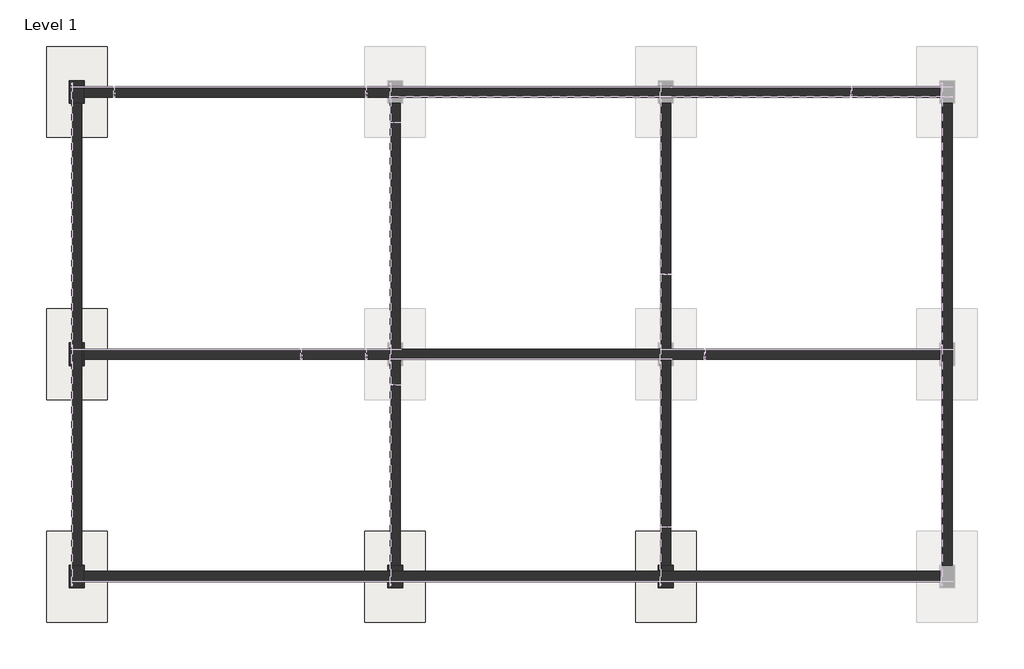
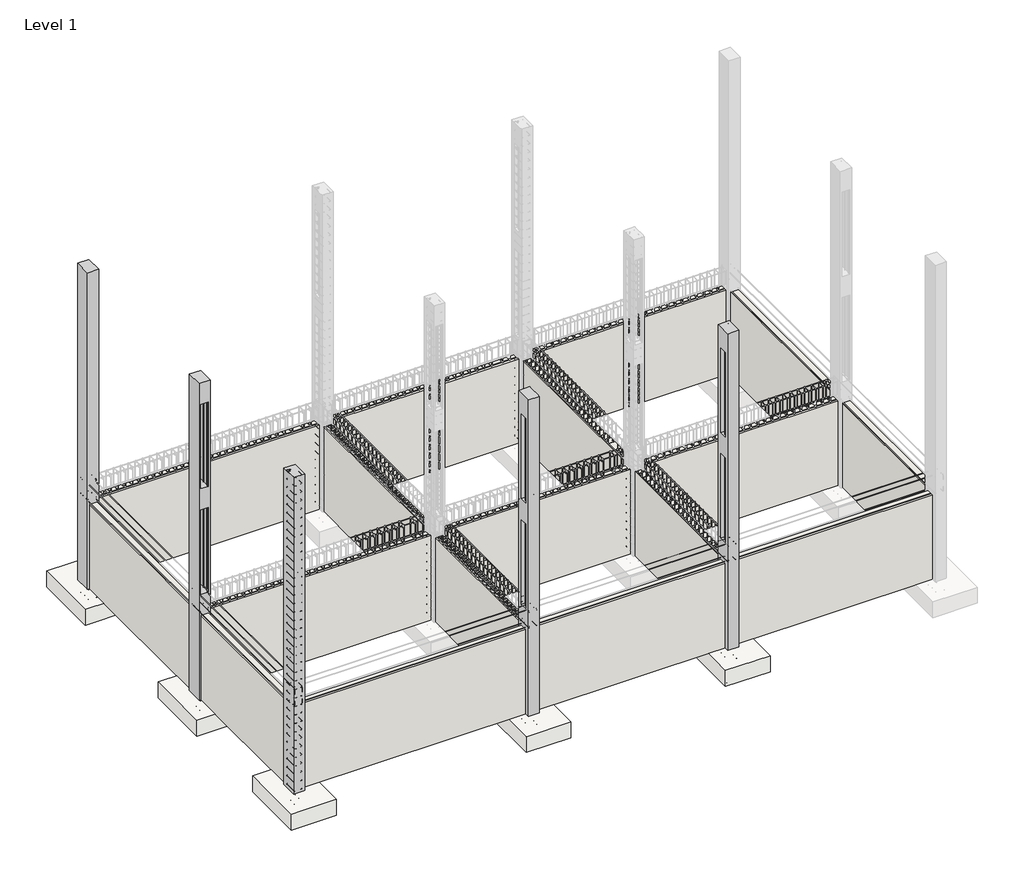
# One storey, part 1 of 8: 7 walls, 5 columns, 5 slabs.
"""IFC4 building model written with IfcOpenShell, lengths in millimetres."""

from ifc_helpers import new_model, si_unit, frame, origin, place, context, project, spatial, polyline, outline, extrude, faceted_brep, element, save

model = new_model("IFC4")

# Units and contexts
model_context = context("Model", 3, world=origin())
ifc_project = project(units=[si_unit("LENGTHUNIT", "METRE", prefix="MILLI")], contexts=[model_context])

# Site, building, storey
site = spatial("IfcSite", under=ifc_project)
building = spatial("IfcBuilding", under=site)
storey = spatial("IfcBuildingStorey", under=building, Name="Level 1", Elevation=0.0)

# Columns
placement = place(None, origin())
element("IfcColumn", 1, ObjectType="Concrete-Rectangular-Column : 12 x 18", at=placement, inside=storey, context=model_context, shape_type="Brep", body=[
    faceted_brep([(-20613.7343089, 13100.2555262, 0.0), (-20613.7343089, 12973.2555262, 0.0), (-20613.7343089, 12770.0555262, 0.0), (-20613.7343089, 12643.0555262, 0.0), (-20664.5343089, 12643.0555262, 0.0), (-20867.7343089, 12643.0555262, 0.0), (-20918.5343089, 12643.0555262, 0.0), (-20918.5343089, 13100.2555262, 0.0), (-20613.7343089, 13100.2555262, 9144.0), (-20613.7343089, 12643.0555262, 9144.0), (-20918.5343089, 12643.0555262, 9144.0), (-20918.5343089, 13100.2555262, 9144.0)], [[[0, 1, 2, 3, 4, 5, 6, 7]], [[8, 9, 3, 2, 1, 0]], [[9, 10, 6, 5, 4, 3]], [[10, 11, 7, 6]], [[11, 8, 0, 7]], [[8, 11, 10, 9]]]),
])
element("IfcColumn", 2, ObjectType="Concrete-Rectangular-Column : 12 x 18", at=placement, inside=storey, context=model_context, shape_type="Brep", body=[
    faceted_brep([(-20918.5343089, 7364.6820829, 0.0), (-20918.5343089, 7821.8820829, 0.0), (-20867.7343089, 7821.8820829, 0.0), (-20867.7343089, 7364.6820829, 0.0), (-20613.7343089, 7364.6820829, 0.0), (-20613.7343089, 7491.6820829, 0.0), (-20613.7343089, 7694.8820829, 0.0), (-20613.7343089, 7821.8820829, 0.0), (-20613.7343089, 7821.8820829, 2438.4), (-20613.7343089, 7821.8820829, 3048.0), (-20613.7343089, 7821.8820829, 5486.4), (-20613.7343089, 7821.8820829, 6096.0), (-20613.7343089, 7821.8820829, 8534.4), (-20613.7343089, 7821.8820829, 9144.0), (-20613.7343089, 7364.6820829, 9144.0), (-20613.7343089, 7364.6820829, 8534.4), (-20613.7343089, 7364.6820829, 6096.0), (-20613.7343089, 7364.6820829, 5486.4), (-20613.7343089, 7364.6820829, 3048.0), (-20613.7343089, 7364.6820829, 2438.4), (-20918.5343089, 7364.6820829, 9144.0), (-20918.5343089, 7364.6820829, 8534.4), (-20918.5343089, 7364.6820829, 6096.0), (-20918.5343089, 7364.6820829, 5486.4), (-20918.5343089, 7364.6820829, 3048.0), (-20918.5343089, 7364.6820829, 2438.4), (-20867.7343089, 7364.6820829, 2438.4), (-20664.5343089, 7364.6820829, 2438.4), (-20664.5343089, 7364.6820829, 0.0), (-20664.5343089, 7364.6820829, 5486.4), (-20664.5343089, 7364.6820829, 3048.0), (-20867.7343089, 7364.6820829, 3048.0), (-20867.7343089, 7364.6820829, 5486.4), (-20664.5343089, 7364.6820829, 8534.4), (-20664.5343089, 7364.6820829, 6096.0), (-20867.7343089, 7364.6820829, 6096.0), (-20867.7343089, 7364.6820829, 8534.4), (-20918.5343089, 7821.8820829, 9144.0), (-20918.5343089, 7821.8820829, 8534.4), (-20918.5343089, 7821.8820829, 6096.0), (-20918.5343089, 7821.8820829, 5486.4), (-20918.5343089, 7821.8820829, 3048.0), (-20918.5343089, 7821.8820829, 2438.4), (-20664.5343089, 7821.8820829, 0.0), (-20664.5343089, 7821.8820829, 2438.4), (-20867.7343089, 7821.8820829, 2438.4), (-20664.5343089, 7821.8820829, 3048.0), (-20664.5343089, 7821.8820829, 5486.4), (-20867.7343089, 7821.8820829, 5486.4), (-20867.7343089, 7821.8820829, 3048.0), (-20664.5343089, 7821.8820829, 6096.0), (-20664.5343089, 7821.8820829, 8534.4), (-20867.7343089, 7821.8820829, 8534.4), (-20867.7343089, 7821.8820829, 6096.0)], [[[0, 1, 2, 3]], [[4, 5, 6, 7, 8, 9, 10, 11, 12, 13, 14, 15, 16, 17, 18, 19]], [[4, 19, 18, 17, 16, 15, 14, 20, 21, 22, 23, 24, 25, 0, 3, 26, 27, 28], [29, 30, 31, 32], [33, 34, 35, 36]], [[1, 0, 25, 24, 23, 22, 21, 20, 37, 38, 39, 40, 41, 42]], [[13, 12, 11, 10, 9, 8, 7, 43, 44, 45, 2, 1, 42, 41, 40, 39, 38, 37], [46, 47, 48, 49], [50, 51, 52, 53]], [[14, 13, 37, 20]], [[43, 28, 27, 44]], [[3, 2, 45, 26]], [[27, 26, 45, 44]], [[7, 6, 5, 4, 28, 43]], [[29, 47, 46, 30]], [[31, 49, 48, 32]], [[30, 46, 49, 31]], [[47, 29, 32, 48]], [[33, 51, 50, 34]], [[35, 53, 52, 36]], [[34, 50, 53, 35]], [[51, 33, 36, 52]]]),
])
element("IfcColumn", 3, ObjectType="Concrete-Rectangular-Column : 12 x 18", at=placement, inside=storey, context=model_context, shape_type="Brep", body=[
    faceted_brep([(-20613.7343089, 3351.1050327, 0.0), (-20613.7343089, 3224.1050327, 0.0), (-20613.7343089, 3020.9050327, 0.0), (-20613.7343089, 2893.9050327, 0.0), (-20918.5343089, 2893.9050327, 0.0), (-20918.5343089, 3351.1050327, 0.0), (-20867.7343089, 3351.1050327, 0.0), (-20664.5343089, 3351.1050327, 0.0), (-20613.7343089, 3351.1050327, 9144.0), (-20613.7343089, 2893.9050327, 9144.0), (-20918.5343089, 2893.9050327, 9144.0), (-20918.5343089, 3351.1050327, 9144.0)], [[[0, 1, 2, 3, 4, 5, 6, 7]], [[8, 9, 3, 2, 1, 0]], [[9, 10, 4, 3]], [[10, 11, 5, 4]], [[11, 8, 0, 7, 6, 5]], [[8, 11, 10, 9]]]),
])
element("IfcColumn", 4, ObjectType="Concrete-Rectangular-Column : 12 x 18", at=placement, inside=storey, context=model_context, shape_type="Brep", body=[
    faceted_brep([(-14513.8601545, 3351.1050327, 0.0), (-14463.0601545, 3351.1050327, 0.0), (-14259.8601545, 3351.1050327, 0.0), (-14209.0601545, 3351.1050327, 0.0), (-14209.0601545, 3224.1050327, 0.0), (-14513.8601545, 3224.1050327, 0.0), (-14209.0601545, 3351.1050327, 9144.0), (-14209.0601545, 3274.9050327, 9144.0), (-14209.0601545, 2970.1050327, 9144.0), (-14209.0601545, 2893.9050327, 9144.0), (-14209.0601545, 2893.9050327, 0.0), (-14209.0601545, 3020.9050327, 0.0), (-14209.0601545, 3020.9050327, 2438.4), (-14209.0601545, 3224.1050327, 2438.4), (-14209.0601545, 3224.1050327, 5486.4), (-14209.0601545, 3224.1050327, 3048.0), (-14209.0601545, 3020.9050327, 3048.0), (-14209.0601545, 3020.9050327, 5486.4), (-14209.0601545, 3224.1050327, 8534.4), (-14209.0601545, 3224.1050327, 6096.0), (-14209.0601545, 3020.9050327, 6096.0), (-14209.0601545, 3020.9050327, 8534.4), (-14513.8601545, 2893.9050327, 0.0), (-14513.8601545, 2893.9050327, 9144.0), (-14513.8601545, 2970.1050327, 9144.0), (-14513.8601545, 3274.9050327, 9144.0), (-14513.8601545, 3351.1050327, 9144.0), (-14513.8601545, 3224.1050327, 2438.4), (-14513.8601545, 3020.9050327, 2438.4), (-14513.8601545, 3020.9050327, 0.0), (-14513.8601545, 3224.1050327, 3048.0), (-14513.8601545, 3224.1050327, 5486.4), (-14513.8601545, 3020.9050327, 5486.4), (-14513.8601545, 3020.9050327, 3048.0), (-14513.8601545, 3224.1050327, 6096.0), (-14513.8601545, 3224.1050327, 8534.4), (-14513.8601545, 3020.9050327, 8534.4), (-14513.8601545, 3020.9050327, 6096.0)], [[[0, 1, 2, 3, 4, 5]], [[6, 7, 8, 9, 10, 11, 12, 13, 4, 3], [14, 15, 16, 17], [18, 19, 20, 21]], [[22, 10, 9, 23]], [[22, 23, 24, 25, 26, 0, 5, 27, 28, 29], [30, 31, 32, 33], [34, 35, 36, 37]], [[3, 2, 1, 0, 26, 6]], [[9, 8, 7, 6, 26, 25, 24, 23]], [[5, 4, 13, 27]], [[11, 29, 28, 12]], [[13, 12, 28, 27]], [[10, 22, 29, 11]], [[14, 31, 30, 15]], [[16, 33, 32, 17]], [[15, 30, 33, 16]], [[31, 14, 17, 32]], [[18, 35, 34, 19]], [[20, 37, 36, 21]], [[19, 34, 37, 20]], [[35, 18, 21, 36]]]),
])
element("IfcColumn", 5, ObjectType="Concrete-Rectangular-Column : 12 x 18", at=placement, inside=storey, context=model_context, shape_type="Brep", body=[
    faceted_brep([(-9068.0732157, 3351.1050327, 0.0), (-9017.2732157, 3351.1050327, 0.0), (-8814.0732157, 3351.1050327, 0.0), (-8763.2732157, 3351.1050327, 0.0), (-8763.2732157, 3224.1050327, 0.0), (-9068.0732157, 3224.1050327, 0.0), (-8763.2732157, 3351.1050327, 9144.0), (-8763.2732157, 3274.9050327, 9144.0), (-8763.2732157, 2970.1050327, 9144.0), (-8763.2732157, 2893.9050327, 9144.0), (-8763.2732157, 2893.9050327, 0.0), (-8763.2732157, 3020.9050327, 0.0), (-8763.2732157, 3020.9050327, 2438.4), (-8763.2732157, 3224.1050327, 2438.4), (-8763.2732157, 3224.1050327, 5486.4), (-8763.2732157, 3224.1050327, 3048.0), (-8763.2732157, 3020.9050327, 3048.0), (-8763.2732157, 3020.9050327, 5486.4), (-8763.2732157, 3224.1050327, 8534.4), (-8763.2732157, 3224.1050327, 6096.0), (-8763.2732157, 3020.9050327, 6096.0), (-8763.2732157, 3020.9050327, 8534.4), (-9068.0732157, 2893.9050327, 0.0), (-9068.0732157, 2893.9050327, 9144.0), (-9068.0732157, 2970.1050327, 9144.0), (-9068.0732157, 3274.9050327, 9144.0), (-9068.0732157, 3351.1050327, 9144.0), (-9068.0732157, 3224.1050327, 2438.4), (-9068.0732157, 3020.9050327, 2438.4), (-9068.0732157, 3020.9050327, 0.0), (-9068.0732157, 3224.1050327, 3048.0), (-9068.0732157, 3224.1050327, 5486.4), (-9068.0732157, 3020.9050327, 5486.4), (-9068.0732157, 3020.9050327, 3048.0), (-9068.0732157, 3224.1050327, 6096.0), (-9068.0732157, 3224.1050327, 8534.4), (-9068.0732157, 3020.9050327, 8534.4), (-9068.0732157, 3020.9050327, 6096.0)], [[[0, 1, 2, 3, 4, 5]], [[6, 7, 8, 9, 10, 11, 12, 13, 4, 3], [14, 15, 16, 17], [18, 19, 20, 21]], [[22, 10, 9, 23]], [[22, 23, 24, 25, 26, 0, 5, 27, 28, 29], [30, 31, 32, 33], [34, 35, 36, 37]], [[3, 2, 1, 0, 26, 6]], [[9, 8, 7, 6, 26, 25, 24, 23]], [[5, 4, 13, 27]], [[11, 29, 28, 12]], [[13, 12, 28, 27]], [[10, 22, 29, 11]], [[14, 31, 30, 15]], [[16, 33, 32, 17]], [[15, 30, 33, 16]], [[31, 14, 17, 32]], [[18, 35, 34, 19]], [[20, 37, 36, 21]], [[19, 34, 37, 20]], [[35, 18, 21, 36]]]),
])

# Slabs
element("IfcSlab", 6, ObjectType="Footing-Rectangular : 72\" x 48\" x 18\"", at=placement, inside=storey, context=model_context, shape_type="SweptSolid", body=[
    extrude(outline(polyline([(-20156.5343089, 13786.0555262), (-20156.5343089, 11957.2555262), (-21375.7343089, 11957.2555262), (-21375.7343089, 13786.0555262), (-20156.5343089, 13786.0555262)])), frame((0.0, 0.0, -457.2), z_axis=(0.0, 0.0, 1.0), x_axis=(1.0, 0.0, 0.0)), (0.0, 0.0, 1.0), 457.2),
])
element("IfcSlab", 7, ObjectType="Footing-Rectangular : 72\" x 48\" x 18\"", at=placement, inside=storey, context=model_context, shape_type="SweptSolid", body=[
    extrude(outline(polyline([(-20156.5343089, 8507.6820829), (-20156.5343089, 6678.8820829), (-21375.7343089, 6678.8820829), (-21375.7343089, 8507.6820829), (-20156.5343089, 8507.6820829)])), frame((0.0, 0.0, -457.2), z_axis=(0.0, 0.0, 1.0), x_axis=(1.0, 0.0, 0.0)), (0.0, 0.0, 1.0), 457.2),
])
element("IfcSlab", 8, ObjectType="Footing-Rectangular : 72\" x 48\" x 18\"", at=placement, inside=storey, context=model_context, shape_type="SweptSolid", body=[
    extrude(outline(polyline([(-20156.5343089, 4036.9050327), (-20156.5343089, 2208.1050327), (-21375.7343089, 2208.1050327), (-21375.7343089, 4036.9050327), (-20156.5343089, 4036.9050327)])), frame((0.0, 0.0, -457.2), z_axis=(0.0, 0.0, 1.0), x_axis=(1.0, 0.0, 0.0)), (0.0, 0.0, 1.0), 457.2),
])
element("IfcSlab", 9, ObjectType="Footing-Rectangular : 72\" x 48\" x 18\"", at=placement, inside=storey, context=model_context, shape_type="SweptSolid", body=[
    extrude(outline(polyline([(-13751.8601545, 4036.9050327), (-13751.8601545, 2208.1050327), (-14971.0601545, 2208.1050327), (-14971.0601545, 4036.9050327), (-13751.8601545, 4036.9050327)])), frame((0.0, 0.0, -457.2), z_axis=(0.0, 0.0, 1.0), x_axis=(1.0, 0.0, 0.0)), (0.0, 0.0, 1.0), 457.2),
])
element("IfcSlab", 10, ObjectType="Footing-Rectangular : 72\" x 48\" x 18\"", at=placement, inside=storey, context=model_context, shape_type="SweptSolid", body=[
    extrude(outline(polyline([(-8306.0732157, 4036.9050327), (-8306.0732157, 2208.1050327), (-9525.2732157, 2208.1050327), (-9525.2732157, 4036.9050327), (-8306.0732157, 4036.9050327)])), frame((0.0, 0.0, -457.2), z_axis=(0.0, 0.0, 1.0), x_axis=(1.0, 0.0, 0.0)), (0.0, 0.0, 1.0), 457.2),
])

# Walls
element("IfcWall", 11, ObjectType="Generic - 8\"", at=placement, inside=storey, context=model_context, shape_type="Brep", body=[
    faceted_brep([(-20613.7343089, 12770.0555262, 0.0), (-14513.8601545, 12770.0555262, 0.0), (-14209.0601545, 12770.0555262, 0.0), (-9068.0732157, 12770.0555262, 0.0), (-8763.2732157, 12770.0555262, 0.0), (-3408.259716, 12770.0555262, 0.0), (-3408.259716, 12770.0555262, 2438.4), (-8763.2732157, 12770.0555262, 2438.4), (-9068.0732157, 12770.0555262, 2438.4), (-14209.0601545, 12770.0555262, 2438.4), (-14513.8601545, 12770.0555262, 2438.4), (-20613.7343089, 12770.0555262, 2438.4), (-20613.7343089, 12973.2555262, 0.0), (-20613.7343089, 12973.2555262, 2438.4), (-14513.8601545, 12973.2555262, 2438.4), (-14209.0601545, 12973.2555262, 2438.4), (-9068.0732157, 12973.2555262, 2438.4), (-8763.2732157, 12973.2555262, 2438.4), (-3408.259716, 12973.2555262, 2438.4), (-3408.259716, 12973.2555262, 0.0), (-8763.2732157, 12973.2555262, 0.0), (-9068.0732157, 12973.2555262, 0.0), (-14209.0601545, 12973.2555262, 0.0), (-14513.8601545, 12973.2555262, 0.0)], [[[0, 1, 2, 3, 4, 5, 6, 7, 8, 9, 10, 11]], [[12, 13, 14, 15, 16, 17, 18, 19, 20, 21, 22, 23]], [[5, 4, 3, 2, 1, 0, 12, 23, 22, 21, 20, 19]], [[6, 5, 19, 18]], [[11, 10, 9, 8, 7, 6, 18, 17, 16, 15, 14, 13]], [[0, 11, 13, 12]]]),
])
element("IfcWall", 12, ObjectType="Generic - 8\"", at=placement, inside=storey, context=model_context, shape_type="Brep", body=[
    faceted_brep([(-3357.459716, 12643.0555262, 0.0), (-3357.459716, 7821.8820829, 0.0), (-3357.459716, 7364.6820829, 0.0), (-3357.459716, 3351.1050327, 0.0), (-3357.459716, 3351.1050327, 2438.4), (-3357.459716, 7364.6820829, 2438.4), (-3357.459716, 7821.8820829, 2438.4), (-3357.459716, 12643.0555262, 2438.4), (-3154.259716, 12643.0555262, 0.0), (-3154.259716, 12643.0555262, 2438.4), (-3154.259716, 7821.8820829, 2438.4), (-3154.259716, 7364.6820829, 2438.4), (-3154.259716, 3351.1050327, 2438.4), (-3154.259716, 3351.1050327, 0.0), (-3154.259716, 7364.6820829, 0.0), (-3154.259716, 7821.8820829, 0.0)], [[[0, 1, 2, 3, 4, 5, 6, 7]], [[8, 9, 10, 11, 12, 13, 14, 15]], [[3, 2, 1, 0, 8, 15, 14, 13]], [[4, 3, 13, 12]], [[7, 6, 5, 4, 12, 11, 10, 9]], [[0, 7, 9, 8]]]),
])
element("IfcWall", 13, ObjectType="Generic - 8\"", at=placement, inside=storey, context=model_context, shape_type="Brep", body=[
    faceted_brep([(-3408.259716, 3224.1050327, 0.0), (-8763.2732157, 3224.1050327, 0.0), (-9068.0732157, 3224.1050327, 0.0), (-14209.0601545, 3224.1050327, 0.0), (-14513.8601545, 3224.1050327, 0.0), (-20613.7343089, 3224.1050327, 0.0), (-20613.7343089, 3224.1050327, 2438.4), (-14513.8601545, 3224.1050327, 2438.4), (-14209.0601545, 3224.1050327, 2438.4), (-9068.0732157, 3224.1050327, 2438.4), (-8763.2732157, 3224.1050327, 2438.4), (-3408.259716, 3224.1050327, 2438.4), (-3408.259716, 3020.9050327, 0.0), (-3408.259716, 3020.9050327, 2438.4), (-8763.2732157, 3020.9050327, 2438.4), (-9068.0732157, 3020.9050327, 2438.4), (-14209.0601545, 3020.9050327, 2438.4), (-14513.8601545, 3020.9050327, 2438.4), (-20613.7343089, 3020.9050327, 2438.4), (-20613.7343089, 3020.9050327, 0.0), (-14513.8601545, 3020.9050327, 0.0), (-14209.0601545, 3020.9050327, 0.0), (-9068.0732157, 3020.9050327, 0.0), (-8763.2732157, 3020.9050327, 0.0)], [[[0, 1, 2, 3, 4, 5, 6, 7, 8, 9, 10, 11]], [[12, 13, 14, 15, 16, 17, 18, 19, 20, 21, 22, 23]], [[5, 4, 3, 2, 1, 0, 12, 23, 22, 21, 20, 19]], [[6, 5, 19, 18]], [[11, 10, 9, 8, 7, 6, 18, 17, 16, 15, 14, 13]], [[0, 11, 13, 12]]]),
])
element("IfcWall", 14, ObjectType="Generic - 8\"", at=placement, inside=storey, context=model_context, shape_type="Brep", body=[
    faceted_brep([(-20664.5343089, 3351.1050327, 0.0), (-20664.5343089, 7364.6820829, 0.0), (-20664.5343089, 7821.8820829, 0.0), (-20664.5343089, 12643.0555262, 0.0), (-20664.5343089, 12643.0555262, 2438.4), (-20664.5343089, 7821.8820829, 2438.4), (-20664.5343089, 7364.6820829, 2438.4), (-20664.5343089, 3351.1050327, 2438.4), (-20867.7343089, 3351.1050327, 0.0), (-20867.7343089, 3351.1050327, 2438.4), (-20867.7343089, 7364.6820829, 2438.4), (-20867.7343089, 7821.8820829, 2438.4), (-20867.7343089, 12643.0555262, 2438.4), (-20867.7343089, 12643.0555262, 0.0), (-20867.7343089, 7821.8820829, 0.0), (-20867.7343089, 7364.6820829, 0.0)], [[[0, 1, 2, 3, 4, 5, 6, 7]], [[8, 9, 10, 11, 12, 13, 14, 15]], [[3, 2, 1, 0, 8, 15, 14, 13]], [[4, 3, 13, 12]], [[7, 6, 5, 4, 12, 11, 10, 9]], [[0, 7, 9, 8]]]),
])
element("IfcWall", 15, ObjectType="Generic - 8\"", at=placement, inside=storey, context=model_context, shape_type="Brep", body=[
    faceted_brep([(-20613.7343089, 7491.6820829, 0.0), (-14513.8601545, 7491.6820829, 0.0), (-14463.0601545, 7491.6820829, 0.0), (-14259.8601545, 7491.6820829, 0.0), (-14209.0601545, 7491.6820829, 0.0), (-9068.0732157, 7491.6820829, 0.0), (-9017.2732157, 7491.6820829, 0.0), (-8814.0732157, 7491.6820829, 0.0), (-8763.2732157, 7491.6820829, 0.0), (-3408.259716, 7491.6820829, 0.0), (-3408.259716, 7491.6820829, 2438.4), (-8763.2732157, 7491.6820829, 2438.4), (-8814.0732157, 7491.6820829, 2438.4), (-9017.2732157, 7491.6820829, 2438.4), (-9068.0732157, 7491.6820829, 2438.4), (-14209.0601545, 7491.6820829, 2438.4), (-14259.8601545, 7491.6820829, 2438.4), (-14463.0601545, 7491.6820829, 2438.4), (-14513.8601545, 7491.6820829, 2438.4), (-20613.7343089, 7491.6820829, 2438.4), (-20613.7343089, 7694.8820829, 0.0), (-20613.7343089, 7694.8820829, 2438.4), (-14513.8601545, 7694.8820829, 2438.4), (-14463.0601545, 7694.8820829, 2438.4), (-14259.8601545, 7694.8820829, 2438.4), (-14209.0601545, 7694.8820829, 2438.4), (-9068.0732157, 7694.8820829, 2438.4), (-9017.2732157, 7694.8820829, 2438.4), (-8814.0732157, 7694.8820829, 2438.4), (-8763.2732157, 7694.8820829, 2438.4), (-3408.259716, 7694.8820829, 2438.4), (-3408.259716, 7694.8820829, 0.0), (-8763.2732157, 7694.8820829, 0.0), (-8814.0732157, 7694.8820829, 0.0), (-9017.2732157, 7694.8820829, 0.0), (-9068.0732157, 7694.8820829, 0.0), (-14209.0601545, 7694.8820829, 0.0), (-14259.8601545, 7694.8820829, 0.0), (-14463.0601545, 7694.8820829, 0.0), (-14513.8601545, 7694.8820829, 0.0)], [[[0, 1, 2, 3, 4, 5, 6, 7, 8, 9, 10, 11, 12, 13, 14, 15, 16, 17, 18, 19]], [[20, 21, 22, 23, 24, 25, 26, 27, 28, 29, 30, 31, 32, 33, 34, 35, 36, 37, 38, 39]], [[9, 8, 7, 6, 5, 4, 3, 2, 1, 0, 20, 39, 38, 37, 36, 35, 34, 33, 32, 31]], [[10, 9, 31, 30]], [[19, 18, 17, 16, 15, 14, 13, 12, 11, 10, 30, 29, 28, 27, 26, 25, 24, 23, 22, 21]], [[0, 19, 21, 20]]]),
])
element("IfcWall", 16, ObjectType="Generic - 8\"", at=placement, inside=storey, context=model_context, shape_type="Brep", body=[
    faceted_brep([(-9017.2732157, 3351.1050327, 0.0), (-9017.2732157, 3351.1050327, 2438.4), (-9017.2732157, 7364.6820829, 2438.4), (-9017.2732157, 7491.6820829, 2438.4), (-9017.2732157, 7491.6820829, 0.0), (-9017.2732157, 7364.6820829, 0.0), (-8814.0732157, 3351.1050327, 2438.4), (-8814.0732157, 3351.1050327, 0.0), (-8814.0732157, 7364.6820829, 0.0), (-8814.0732157, 7491.6820829, 0.0), (-8814.0732157, 7491.6820829, 2438.4), (-8814.0732157, 7364.6820829, 2438.4)], [[[0, 1, 2, 3, 4, 5]], [[6, 7, 8, 9, 10, 11]], [[7, 0, 5, 4, 9, 8]], [[1, 0, 7, 6]], [[1, 6, 11, 10, 3, 2]], [[4, 3, 10, 9]]]),
    faceted_brep([(-9017.2732157, 12643.0555262, 2438.4), (-9017.2732157, 12643.0555262, 0.0), (-9017.2732157, 7821.8820829, 0.0), (-9017.2732157, 7694.8820829, 0.0), (-9017.2732157, 7694.8820829, 2438.4), (-9017.2732157, 7821.8820829, 2438.4), (-8814.0732157, 12643.0555262, 0.0), (-8814.0732157, 12643.0555262, 2438.4), (-8814.0732157, 7821.8820829, 2438.4), (-8814.0732157, 7694.8820829, 2438.4), (-8814.0732157, 7694.8820829, 0.0), (-8814.0732157, 7821.8820829, 0.0)], [[[0, 1, 2, 3, 4, 5]], [[6, 7, 8, 9, 10, 11]], [[1, 6, 11, 10, 3, 2]], [[7, 0, 5, 4, 9, 8]], [[1, 0, 7, 6]], [[4, 3, 10, 9]]]),
])
element("IfcWall", 17, ObjectType="Generic - 8\"", at=placement, inside=storey, context=model_context, shape_type="Brep", body=[
    faceted_brep([(-14259.8601545, 12643.0555262, 0.0), (-14259.8601545, 12643.0555262, 2438.4), (-14259.8601545, 7821.8820829, 2438.4), (-14259.8601545, 7694.8820829, 2438.4), (-14259.8601545, 7694.8820829, 0.0), (-14259.8601545, 7821.8820829, 0.0), (-14463.0601545, 12643.0555262, 2438.4), (-14463.0601545, 12643.0555262, 0.0), (-14463.0601545, 7821.8820829, 0.0), (-14463.0601545, 7694.8820829, 0.0), (-14463.0601545, 7694.8820829, 2438.4), (-14463.0601545, 7821.8820829, 2438.4)], [[[0, 1, 2, 3, 4, 5]], [[6, 7, 8, 9, 10, 11]], [[7, 0, 5, 4, 9, 8]], [[1, 0, 7, 6]], [[1, 6, 11, 10, 3, 2]], [[4, 3, 10, 9]]]),
    faceted_brep([(-14259.8601545, 3351.1050327, 2438.4), (-14259.8601545, 3351.1050327, 0.0), (-14259.8601545, 7364.6820829, 0.0), (-14259.8601545, 7491.6820829, 0.0), (-14259.8601545, 7491.6820829, 2438.4), (-14259.8601545, 7364.6820829, 2438.4), (-14463.0601545, 3351.1050327, 0.0), (-14463.0601545, 3351.1050327, 2438.4), (-14463.0601545, 7364.6820829, 2438.4), (-14463.0601545, 7491.6820829, 2438.4), (-14463.0601545, 7491.6820829, 0.0), (-14463.0601545, 7364.6820829, 0.0)], [[[0, 1, 2, 3, 4, 5]], [[6, 7, 8, 9, 10, 11]], [[1, 6, 11, 10, 3, 2]], [[7, 0, 5, 4, 9, 8]], [[1, 0, 7, 6]], [[4, 3, 10, 9]]]),
])

save(model, "model.ifc")

# Revit data of these elements
# Type "Concrete-Rectangular-Column : 12 x 18"
#   Assembly Code = "B10"
#   b = 1' - 0"
#   h = 1' - 6"
#   Structural Material [instance default] = Concrete, Cast-in-Place gray
# Type "Footing-Rectangular : 72\" x 48\" x 18\""
#   Assembly Code = "A1010100"
#   Width = 4' - 0"
#   Length = 6' - 0"
#   Foundation Thickness = 1' - 6"
#   Structural Material [instance default] = Concrete, Cast-in-Place gray
# Type "Generic - 8\""
#   Assembly Code = "B2010"
#   Layers, outside or top first: 0' - 8" no material (function 1)
# Elements 1, 2, 3, 4, 5 (IfcColumn, "Concrete-Rectangular-Column : 12 x 18")
#   Structural Material = Concrete, Cast-in-Place gray
#   Phase Created = New Construction
#   Materials on its faces: "Concrete, Cast-in-Place gray"
# Elements 6, 7, 8, 9, 10 (IfcSlab, "Footing-Rectangular : 72\" x 48\" x 18\"")
#   Structural Material = Concrete, Cast-in-Place gray
#   Phase Created = New Construction
#   Materials on its faces: "Concrete, Cast-in-Place gray"
# Elements 11, 12, 13, 14, 15, 16, 17 (IfcWall, "Generic - 8\"")
#   Top Offset = -2' - 0"
#   Base Offset = 0' - 0"
#   wall height = 8' - 0"
#   Phase Created = New Construction
#   Base Constraint = Level 1
#   Top Constraint = Level 2
#   Materials on its faces: "Default Wall"
# Materials
#   "Concrete, Cast-in-Place gray": class "Concrete", colour RGB 192 192 192, transparency 0, Description = "Cast-in-place concrete", Cost = 0
#   "Default Wall": colour RGB 128 128 128, transparency 0, Cost = 0
